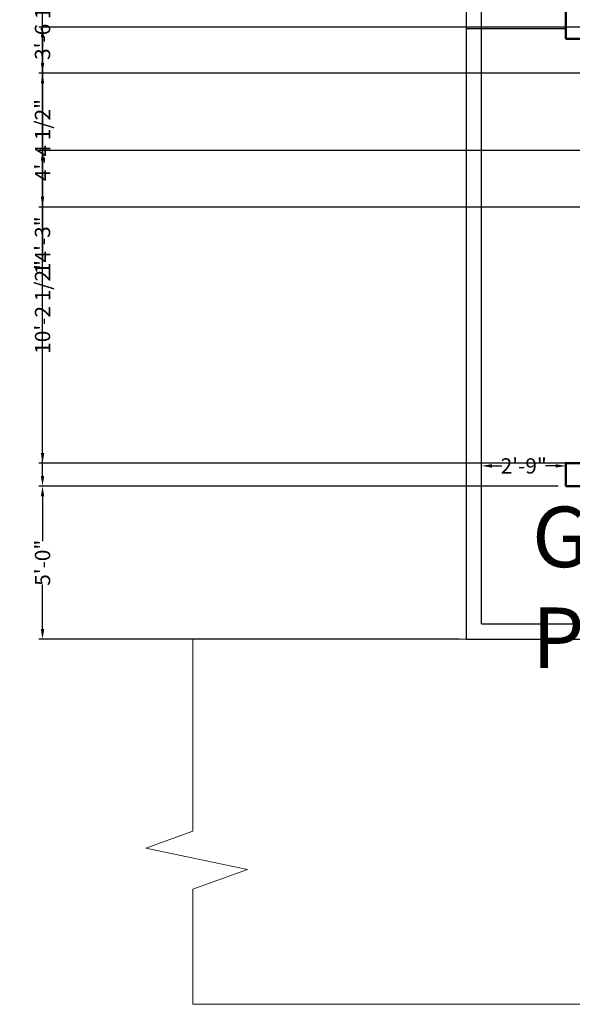
# Model space of a CAD drawing. Units: inches. Extents: x 6704 to 7574, y 11759 to 12617.
# Tile 1 of 8: x 6704 to 6921, y 11809 to 12195. Entities that reach past the tile are written whole.
import ezdxf

# ---------------------------------------------------------------- set-up
doc = ezdxf.new("R2010")
doc.units = ezdxf.units.IN
doc.header["$MEASUREMENT"] = 0
for name, color, linetype, lineweight in [('A-ANNO-SYMB', 8, 'Continuous', 18), ('A-ANNO-TEXT', 7, 'Continuous', 25), ('C-PROP', 7, 'Continuous', 30), ('C-ROAD', 8, 'Continuous', 20), ('WALL', 7, 'Continuous', 50), ('YQ_DIM', 3, 'Continuous', 18)]:
    doc.layers.add(name, color=color, linetype=linetype, lineweight=lineweight)
doc.styles.get("Standard").update_dxf_attribs({"font": 'arial.ttf'})
doc.styles.add('YQ_DIM', font='SUPEROS.SHX', dxfattribs={"width": 0.8, "bigfont": 'HZDX.SHX'})
doc.dimstyles.new('yqi0', dxfattribs={"dimscale": 0, "dimtxt": 6, "dimasz": 4, "dimexe": 1.5, "dimexo": 3, "dimgap": 0.5, "dimtad": 0, "dimdsep": 46, "dimlunit": 4, "dimtxsty": 'Standard', "dimcen": 0, "dimclrd": 256, "dimclre": 256, "dimclrt": 7, "dimadec": 1, "dimazin": 2, "dimtfac": 1, "dimtix": 1, "dimtmove": 2, "dimatfit": 2, "dimfxl": 1, "dimtolj": 1, "dimtzin": 0, "dimarcsym": 0})

# ---------------------------------------------------------------- blocks, each defined once
blk = doc.blocks.new('*D7')
at = {"layer": 'Defpoints', "color": 0, "transparency": 16777216}
for p in [(6885.07, 12019.74), (6885.07, 12011.76), (6918.07, 12011.76)]:
    blk.add_point(p, dxfattribs=at)
at = {"layer": 'YQ_DIM', "color": 0, "lineweight": -2, "transparency": 16777216}
for p, q in [((6885.07, 12014.76), (6885.07, 12021.24)), ((6889.07, 12019.74), (6893.05, 12019.74)), ((6914.07, 12019.74), (6910.1, 12019.74)), ((6918.07, 12014.76), (6918.07, 12021.24))]:
    blk.add_line(p, q, dxfattribs=at)
at = {"layer": 'YQ_DIM', "color": 0, "transparency": 16777216}
for points in [[(6889.07, 12020.41), (6889.07, 12019.07), (6885.07, 12019.74)], [(6914.07, 12020.41), (6914.07, 12019.07), (6918.07, 12019.74)]]:
    blk.add_solid(points, dxfattribs=at)
at = {"layer": 'YQ_DIM', "color": 0, "transparency": 16777216, "insert": (6901.57, 12019.74), "char_height": 6, "attachment_point": 5}
blk.add_mtext('\\A1;2\'-9"', dxfattribs=at)
blk = doc.blocks.new('ROAD-BREAK')
blk.add_lwpolyline([(18.36, 29.8), (18.36, 24.82), (0, 18.15), (39.74, 9.9), (18.36, 2.15), (18.36, 0)])
blk = doc.blocks.new('*D56')
at = {"layer": 'Defpoints', "color": 0, "transparency": 16777216}
for p in [(6712.97, 12511.26), (6918.07, 12511.26), (6918.07, 12011.76)]:
    blk.add_point(p, dxfattribs=at)
at = {"layer": 'YQ_DIM', "lineweight": -2, "transparency": 16777216}
for p, q in [((6915.07, 12511.26), (6711.47, 12511.26)), ((6712.97, 12507.26), (6712.97, 12279.42)), ((6712.97, 12015.76), (6712.97, 12243.59)), ((6915.07, 12011.76), (6711.47, 12011.76))]:
    blk.add_line(p, q, dxfattribs=at)
at = {"layer": 'YQ_DIM', "transparency": 16777216}
for points in [[(6712.3, 12507.26), (6713.64, 12507.26), (6712.97, 12511.26)], [(6712.3, 12015.76), (6713.64, 12015.76), (6712.97, 12011.76)]]:
    blk.add_solid(points, dxfattribs=at)
at = {"layer": 'YQ_DIM', "color": 7, "transparency": 16777216, "insert": (6712.97, 12261.51), "char_height": 6, "attachment_point": 5, "rotation": 90}
blk.add_mtext('\\A1;41\'-7 1/2"', dxfattribs=at)
blk = doc.blocks.new('*D66')
at = {"layer": 'Defpoints', "color": 0, "transparency": 16777216}
for p in [(6712.97, 12173.76), (7062.07, 12173.76), (7062.07, 12121.26)]:
    blk.add_point(p, dxfattribs=at)
at = {"layer": 'YQ_DIM', "lineweight": -2, "transparency": 16777216}
for p, q in [((7059.07, 12173.76), (6711.47, 12173.76)), ((6712.97, 12169.76), (6712.97, 12163.09)), ((6712.97, 12125.26), (6712.97, 12131.92)), ((7059.07, 12121.26), (6711.47, 12121.26))]:
    blk.add_line(p, q, dxfattribs=at)
at = {"layer": 'YQ_DIM', "transparency": 16777216}
for points in [[(6712.3, 12169.76), (6713.64, 12169.76), (6712.97, 12173.76)], [(6712.3, 12125.26), (6713.64, 12125.26), (6712.97, 12121.26)]]:
    blk.add_solid(points, dxfattribs=at)
at = {"layer": 'YQ_DIM', "color": 7, "transparency": 16777216, "insert": (6712.97, 12147.51), "char_height": 6, "attachment_point": 5, "rotation": 90}
blk.add_mtext('\\A1;4\'-4 1/2"', dxfattribs=at)
blk = doc.blocks.new('*D71')
at = {"layer": 'Defpoints', "color": 0, "transparency": 16777216}
for p in [(6918.07, 12011.76), (6712.97, 11951.76), (6879.07, 11951.76)]:
    blk.add_point(p, dxfattribs=at)
at = {"layer": 'YQ_DIM', "lineweight": -2, "transparency": 16777216}
for p, q in [((6915.07, 12011.76), (6711.47, 12011.76)), ((6712.97, 12007.76), (6712.97, 11990.23)), ((6712.97, 11955.76), (6712.97, 11973.28)), ((6876.07, 11951.76), (6711.47, 11951.76))]:
    blk.add_line(p, q, dxfattribs=at)
at = {"layer": 'YQ_DIM', "transparency": 16777216}
for points in [[(6712.3, 12007.76), (6713.64, 12007.76), (6712.97, 12011.76)], [(6712.3, 11955.76), (6713.64, 11955.76), (6712.97, 11951.76)]]:
    blk.add_solid(points, dxfattribs=at)
at = {"layer": 'YQ_DIM', "color": 7, "transparency": 16777216, "insert": (6712.97, 11981.76), "char_height": 6, "attachment_point": 5, "rotation": 90}
blk.add_mtext('\\A1;5\'-0"', dxfattribs=at)
blk = doc.blocks.new('*D74')
at = {"layer": 'Defpoints', "color": 0, "transparency": 16777216}
for p in [(6712.97, 12191.76), (6948.07, 12191.76), (6948.07, 12020.76)]:
    blk.add_point(p, dxfattribs=at)
at = {"layer": 'YQ_DIM', "lineweight": -2, "transparency": 16777216}
for p, q in [((6945.07, 12191.76), (6711.47, 12191.76)), ((6712.97, 12187.76), (6712.97, 12116.78)), ((6712.97, 12024.76), (6712.97, 12095.73)), ((6945.07, 12020.76), (6711.47, 12020.76))]:
    blk.add_line(p, q, dxfattribs=at)
at = {"layer": 'YQ_DIM', "transparency": 16777216}
for points in [[(6712.3, 12187.76), (6713.64, 12187.76), (6712.97, 12191.76)], [(6712.3, 12024.76), (6713.64, 12024.76), (6712.97, 12020.76)]]:
    blk.add_solid(points, dxfattribs=at)
at = {"layer": 'YQ_DIM', "color": 7, "transparency": 16777216, "insert": (6712.97, 12106.26), "char_height": 6, "attachment_point": 5, "rotation": 90}
blk.add_mtext('\\A1;14\'-3"', dxfattribs=at)
blk = doc.blocks.new('*D77')
at = {"layer": 'Defpoints', "color": 0, "transparency": 16777216}
for p in [(7260.07, 12216.3), (6712.97, 12173.76), (7260.07, 12173.76)]:
    blk.add_point(p, dxfattribs=at)
at = {"layer": 'YQ_DIM', "lineweight": -2, "transparency": 16777216}
for p, q in [((7257.07, 12216.3), (6711.47, 12216.3)), ((6712.97, 12212.3), (6712.97, 12210.49)), ((6712.97, 12177.76), (6712.97, 12179.57)), ((7257.07, 12173.76), (6711.47, 12173.76))]:
    blk.add_line(p, q, dxfattribs=at)
at = {"layer": 'YQ_DIM', "transparency": 16777216}
for points in [[(6712.3, 12212.3), (6713.64, 12212.3), (6712.97, 12216.3)], [(6712.3, 12177.76), (6713.64, 12177.76), (6712.97, 12173.76)]]:
    blk.add_solid(points, dxfattribs=at)
at = {"layer": 'YQ_DIM', "color": 7, "transparency": 16777216, "insert": (6712.97, 12195.03), "char_height": 6, "attachment_point": 5, "rotation": 90}
blk.add_mtext('\\A1;3\'-6 1/2"', dxfattribs=at)
blk = doc.blocks.new('*D80')
at = {"layer": 'Defpoints', "color": 0, "transparency": 16777216}
for p in [(6712.97, 12143.38), (6948.07, 12143.38), (6948.07, 12020.76)]:
    blk.add_point(p, dxfattribs=at)
at = {"layer": 'YQ_DIM', "lineweight": -2, "transparency": 16777216}
for p, q in [((6945.07, 12143.38), (6711.47, 12143.38)), ((6712.97, 12139.38), (6712.97, 12099.58)), ((6712.97, 12024.76), (6712.97, 12064.56)), ((6945.07, 12020.76), (6711.47, 12020.76))]:
    blk.add_line(p, q, dxfattribs=at)
at = {"layer": 'YQ_DIM', "transparency": 16777216}
for points in [[(6712.3, 12139.38), (6713.64, 12139.38), (6712.97, 12143.38)], [(6712.3, 12024.76), (6713.64, 12024.76), (6712.97, 12020.76)]]:
    blk.add_solid(points, dxfattribs=at)
at = {"layer": 'YQ_DIM', "color": 7, "transparency": 16777216, "insert": (6712.97, 12082.07), "char_height": 6, "attachment_point": 5, "rotation": 90}
blk.add_mtext('\\A1;10\'-2 1/2"', dxfattribs=at)

msp = doc.modelspace()

# ---------------------------------------------------------------- linework, layer by layer
at = {"layer": 'C-PROP'}
for p, q in [((6879.073, 11951.757), (6879.073, 12550.257)), ((6885.073, 11957.757), (6885.073, 12544.257)), ((6918.073, 12191.093), (6879.073, 12191.093)), ((6885.073, 11957.757), (7104.073, 11957.757)), ((6879.073, 11951.757), (7104.073, 11951.757))]:
    msp.add_line(p, q, dxfattribs=at)
at = {"layer": 'C-ROAD'}
for p, q in [((6771.883, 11951.757), (7503.792, 11951.757)), ((6771.883, 11951.757), (6771.883, 11876.472)), ((6771.883, 11853.793), (6771.883, 11808.627)), ((6771.883, 11808.627), (7503.792, 11808.627))]:
    msp.add_line(p, q, dxfattribs=at)
at = {"layer": 'WALL'}
for p, q in [((6918.073, 12187.257), (6918.073, 12284.383)), ((6939.073, 12187.257), (6918.073, 12187.257)), ((6918.073, 12020.757), (6939.073, 12020.757)), ((6918.073, 12020.757), (6918.073, 12011.757)), ((6918.073, 12011.757), (7000.573, 12011.757))]:
    msp.add_line(p, q, dxfattribs=at)

# ---------------------------------------------------------------- block references
at = {"layer": 'A-ANNO-SYMB'}
msp.add_blockref('ROAD-BREAK', (6753.52, 11851.647), dxfattribs=at)

# ---------------------------------------------------------------- texts
at = {"layer": 'A-ANNO-TEXT', "insert": (6904.802, 12003.787), "char_height": 23.74016, "width": 221.66005, "attachment_point": 1, "style": 'YQ_DIM'}
msp.add_mtext('Ground Floor Plan', dxfattribs=at)

# ---------------------------------------------------------------- dimensions: what is measured, and where the dimension line sits
at = {"layer": 'YQ_DIM'}
for base, p1, p2, picture, middle in [((6712.97, 12511.257), (6918.073, 12011.757), (6918.073, 12511.257), '*D56', (6712.97, 12261.507)), ((6712.97, 12173.757), (7260.073, 12216.302), (7260.073, 12173.757), '*D77', (6712.97, 12195.029)), ((6712.97, 12191.757), (6948.073, 12020.757), (6948.073, 12191.757), '*D74', (6712.97, 12106.257)), ((6712.97, 12173.757), (7062.073, 12121.257), (7062.073, 12173.757), '*D66', (6712.97, 12147.507)), ((6712.97, 12143.383), (6948.073, 12020.757), (6948.073, 12143.383), '*D80', (6712.97, 12082.07)), ((6712.97, 11951.757), (6918.073, 12011.757), (6879.073, 11951.757), '*D71', (6712.97, 11981.757))]:
    dim = msp.add_linear_dim(base=base, p1=p1, p2=p2, angle=90, dimstyle='yqi0', override={"dimscale": 1, "dimdec": 1, "dimzin": 1, "dimfrac": 2}, dxfattribs=at)
    dim.commit()
    dim.dimension.update_dxf_attribs({"geometry": picture, "text_midpoint": middle})
dim = msp.add_aligned_dim(p1=(6918.073, 12011.757), p2=(6885.073, 12011.757), distance=-7.982, dimstyle='yqi0', override={"dimscale": 1, "dimclrd": 0, "dimclre": 0, "dimclrt": 0}, dxfattribs=at)
dim.commit()
dim.dimension.update_dxf_attribs({"geometry": '*D7', "text_midpoint": (6901.573, 12019.74)})

doc.saveas('drawing.dxf')
